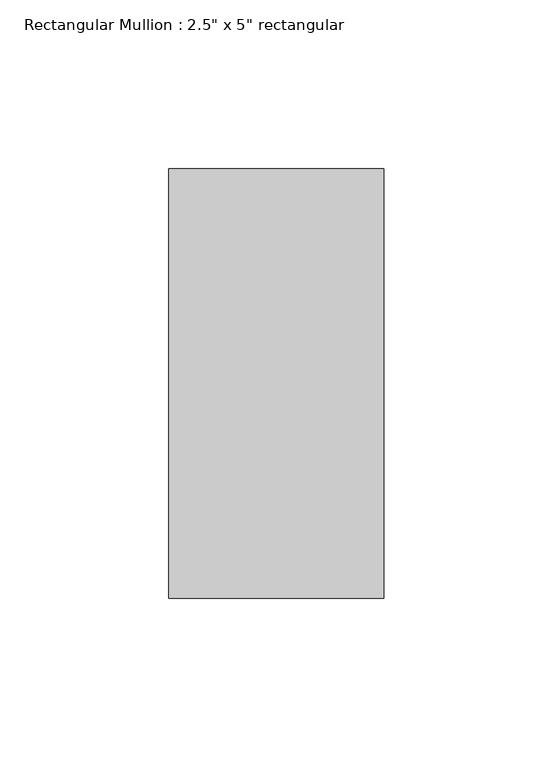
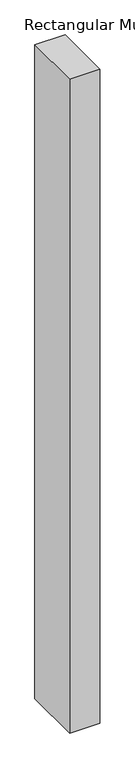
"""IFC4 building model written with IfcOpenShell, lengths in millimetres: member geometry."""

from ifc_helpers import new_model, si_unit, frame, origin, place, context, project, spatial, polyline, outline, extrude, source, transform, mapped, element, save


def member_ead4612c(model_context):
    return source(origin(), model_context, "Body", "SweptSolid", [
        extrude(outline(polyline([(0.0, 63.5), (0.0, -63.5), (-63.5, -63.5), (-63.5, 63.5), (0.0, 63.5)])), frame((0.0, 0.0, -1457.6985165), z_axis=(0.0, 0.0, 1.0), x_axis=(1.0, 0.0, 0.0)), (0.0, 0.0, 1.0), 1457.6985165),
    ])


if __name__ == "__main__":
    model = new_model("IFC4")
    model_context = context("Model", 3, world=origin())
    ifc_project = project(units=[si_unit("LENGTHUNIT", "METRE", prefix="MILLI")], contexts=[model_context])
    site = spatial("IfcSite", under=ifc_project)
    building = spatial("IfcBuilding", under=site)
    placement = place(None, origin())
    member_shape = member_ead4612c(model_context)
    element("IfcMember", 1, ObjectType="Rectangular Mullion : 2.5\" x 5\" rectangular", at=placement, inside=building, context=model_context, shape_type="MappedRepresentation", body=[
        mapped(member_shape, transform((0.0, 0.0, 0.0), x_axis=(1.0, 0.0, 0.0), y_axis=(0.0, 1.0, 0.0), z_axis=(0.0, 0.0, 1.0))),
    ])
    save(model, "model.ifc")

# Revit data of these elements
# Type "Rectangular Mullion : 2.5\" x 5\" rectangular"
#   built-in parameter 1007304 = 0.416667 (stored number, unit not read)
#   built-in parameter 1007301 = 0.104167 (stored number, unit not read)
#   built-in parameter 1007300 = 0.104167 (stored number, unit not read)
# Element 1 (IfcMember, "Rectangular Mullion : 2.5\" x 5\" rectangular")
#   Materials on its faces: "Aluminum"
# Materials
#   "Aluminum": class "Metal", colour RGB 247 247 247, transparency 0, Description = "Aluminum 6061", Cost = 0
